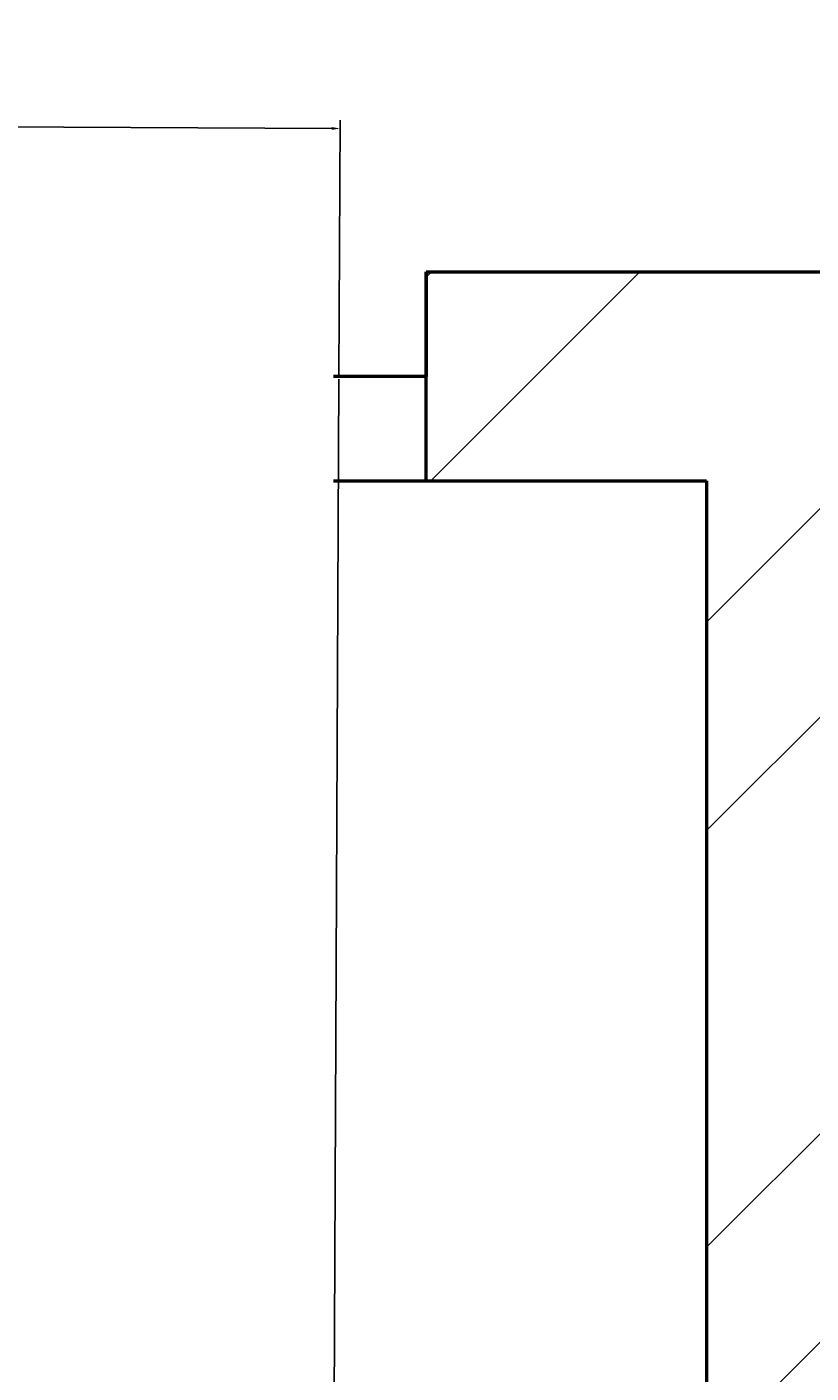
# Model space of a CAD drawing. Units: inches. Extents: x 1901 to 2863, y 888 to 2433.
# Tile 31 of 91: x 2590 to 2607, y 1376 to 1405. Entities that reach past the tile are written whole.
import ezdxf

# ---------------------------------------------------------------- set-up
doc = ezdxf.new("R2010")
doc.units = ezdxf.units.IN
for name, color, linetype, lineweight in [('A-ANNO-DIMS', 2, 'Continuous', 18), ('A-DOOR', 4, 'Continuous', 25), ('A-WALL', 7, 'Continuous', 50), ('A-WALL-PATT', 8, 'Continuous', 13)]:
    doc.layers.add(name, color=color, linetype=linetype, lineweight=lineweight)
doc.styles.get("Standard").update_dxf_attribs({"font": 'arial.ttf'})
doc.dimstyles.get("Standard").update_dxf_attribs({"dimtxt": 0.18, "dimasz": 0.18, "dimexe": 0.18, "dimexo": 0.0625, "dimgap": 0.09, "dimtad": 0, "dimtih": 1, "dimtoh": 1, "dimdec": 4, "dimzin": 0, "dimdsep": 46, "dimtxsty": 'Standard', "dimcen": 0.09, "dimadec": 0, "dimazin": 0, "dimtfac": 1, "dimtdec": 4, "dimtofl": 0, "dimtmove": 0, "dimatfit": 3, "dimfxl": 1, "dimtolj": 1, "dimtzin": 0, "dimarcsym": 0})

# ---------------------------------------------------------------- blocks, each defined once
blk = doc.blocks.new('DOOR-29')
blk.add_line((-0.004, -0.016), (-0.004, 35.984))
blk.add_arc((-0.004, 7.119), 28.865, 345.6888, 90)
blk = doc.blocks.new('*D32')
at = {"layer": 'A-ANNO-DIMS', "color": 0, "lineweight": -2, "transparency": 16777216}
for p, q in [((2566.833, 1398.027), (2566.858, 1403.544)), ((2567.038, 1403.364), (2581.416, 1403.297)), ((2596.85, 1403.225), (2582.472, 1403.292)), ((2597.005, 1397.887), (2597.03, 1403.404))]:
    blk.add_line(p, q, dxfattribs=at)
at = {"layer": 'A-ANNO-DIMS', "color": 0, "transparency": 16777216}
for points in [[(2567.038, 1403.394), (2567.037, 1403.334), (2566.858, 1403.364)], [(2596.85, 1403.255), (2596.849, 1403.195), (2597.03, 1403.224)]]:
    blk.add_solid(points, dxfattribs=at)
at = {"layer": 'Defpoints', "color": 0, "transparency": 16777216}
for p in [(2566.858, 1403.364), (2566.833, 1397.964), (2597.005, 1397.824)]:
    blk.add_point(p, dxfattribs=at)
at = {"layer": 'A-ANNO-DIMS', "color": 0, "transparency": 16777216, "insert": (2581.944, 1403.294), "char_height": 0.18, "attachment_point": 5}
blk.add_mtext('\\A1;30 TYP.', dxfattribs=at)

msp = doc.modelspace()

# ---------------------------------------------------------------- hatches: boundary and pattern name
at = {"layer": 'A-WALL-PATT'}
h = msp.add_hatch(dxfattribs=at)
h.set_pattern_fill('ANSI32', color=256)
h.paths.add_polyline_path([(2443.926, 2139.888), (2439.426, 2139.888), (2439.426, 2069.348), (2441.676, 2069.348), (2443.926, 2069.348), (2443.926, 2078.634), (2521.926, 2078.634), (2521.926, 2075.067), (2524.176, 2075.067), (2526.426, 2075.067), (2526.426, 2078.634), (2571.755, 2078.634), (2571.755, 2080.884), (2571.755, 2083.134), (2443.926, 2083.134)])
h.paths.add_polyline_path([(2526.426, 2054.634), (2524.176, 2054.634), (2521.926, 2054.634), (2521.926, 2030.634), (2443.926, 2030.634), (2443.926, 2045.348), (2439.426, 2045.348), (2439.426, 1983.867), (2443.926, 1983.867), (2443.926, 2026.134), (2521.926, 2026.134), (2526.426, 2026.134)])
h.paths.add_polyline_path([(2443.926, 1923.867), (2439.426, 1923.867), (2439.426, 1872.634), (2443.926, 1872.634)])
h.paths.add_polyline_path([(2636.233, 1766.134), (2609.926, 1766.134), (2609.926, 1779.785), (2605.426, 1779.785), (2605.426, 1766.134), (2486.614, 1766.134), (2486.614, 1770.671), (2482.114, 1770.671), (2482.114, 1766.134), (2482.114, 1761.634), (2636.233, 1761.634), (2636.233, 1763.884)])
h.paths.add_polyline_path([(2519.536, 1663.384), (2519.536, 1665.634), (2494.926, 1665.634), (2481.831, 1665.634), (2481.831, 1663.384), (2481.831, 1661.134), (2490.426, 1661.134), (2490.426, 1640.157), (2494.926, 1640.157), (2494.926, 1661.134), (2519.536, 1661.134)])
h.paths.add_polyline_path([(2443.926, 1712.134), (2443.926, 1716.634), (2414.464, 1716.634), (2414.464, 1712.134), (2439.426, 1712.134), (2439.426, 1545.507), (2443.926, 1545.507), (2443.926, 1661.134), (2448.475, 1661.134), (2448.475, 1665.634), (2443.926, 1665.634)])
h.paths.add_polyline_path([(2343.426, 1712.134), (2365.525, 1712.134), (2365.525, 1714.384), (2365.525, 1716.634), (2333.871, 1716.634), (2333.871, 1714.384), (2333.871, 1712.134), (2338.926, 1712.134), (2338.926, 1575.634), (2338.926, 1545.507), (2343.426, 1545.507), (2343.426, 1547.507), (2343.426, 1580.134)])
h.paths.add_polyline_path([(2752.926, 1665.634), (2579.536, 1665.634), (2579.536, 1661.134), (2615.926, 1661.134), (2615.926, 1529.134), (2598.931, 1529.134), (2598.931, 1524.634), (2623.127, 1524.634), (2623.127, 1526.884), (2623.127, 1529.134), (2620.426, 1529.134), (2620.426, 1661.134), (2748.426, 1661.134), (2748.426, 1633.499), (2752.926, 1633.499)])
h.paths.add_polyline_path([(2752.926, 1419.929), (2748.426, 1419.929), (2748.426, 1400.134), (2659.426, 1400.134), (2659.426, 1444.333), (2657.176, 1444.333), (2654.926, 1444.333), (2654.926, 1400.134), (2643.649, 1400.134), (2643.649, 1395.634), (2748.426, 1395.634), (2748.426, 1364.035), (2752.926, 1364.035)])
h.paths.add_polyline_path([(2752.926, 1492.878), (2748.426, 1492.878), (2748.426, 1476.634), (2667.426, 1476.634), (2667.426, 1479.71), (2665.176, 1479.71), (2662.926, 1479.71), (2662.926, 1476.634), (2654.926, 1476.634), (2654.926, 1469.536), (2659.426, 1469.536), (2659.426, 1472.134), (2748.426, 1472.134), (2748.426, 1455.929), (2752.926, 1455.929)])
h.paths.add_polyline_path([(2752.926, 1304.035), (2748.426, 1304.035), (2748.426, 1263.634), (2738.66, 1263.634), (2738.66, 1259.134), (2752.926, 1259.134)])
h.paths.add_polyline_path([(2685.926, 1259.134), (2695.49, 1259.134), (2695.49, 1261.384), (2695.49, 1263.634), (2677.837, 1263.634), (2677.837, 1261.384), (2677.837, 1259.134), (2681.426, 1259.134), (2681.426, 1203.634), (2653.277, 1203.634), (2653.277, 1199.134), (2685.926, 1199.134), (2685.926, 1203.634)])
h.paths.add_polyline_path([(2609.426, 1395.634), (2611.848, 1395.634), (2611.848, 1400.134), (2598.888, 1400.134), (2598.888, 1397.884), (2598.888, 1395.634), (2604.926, 1395.634), (2604.926, 1268.134), (2554.726, 1268.134), (2554.726, 1265.884), (2554.726, 1263.634), (2604.926, 1263.634), (2604.926, 1203.634), (2571.306, 1203.634), (2571.306, 1199.134), (2604.926, 1199.134), (2629.277, 1199.134), (2629.277, 1201.384), (2629.277, 1203.634), (2609.426, 1203.634), (2609.426, 1258.634), (2609.426, 1259.134), (2654.804, 1259.134), (2654.804, 1263.634), (2609.426, 1263.634)])
h.paths.add_polyline_path([(2443.926, 1304.035), (2439.426, 1304.035), (2439.426, 1259.134), (2443.926, 1259.134), (2456.16, 1259.134), (2456.16, 1261.384), (2456.16, 1263.634), (2443.926, 1263.634)])
h.paths.add_polyline_path([(2525.426, 1263.634), (2531.778, 1263.634), (2531.778, 1268.134), (2520.926, 1268.134), (2520.926, 1263.634), (2511.409, 1263.634), (2511.409, 1259.134), (2520.926, 1259.134), (2520.926, 1199.134), (2547.306, 1199.134), (2547.306, 1201.384), (2547.306, 1203.634), (2525.426, 1203.634)])
h.paths.add_polyline_path([(2443.926, 1434.842), (2439.426, 1434.842), (2439.426, 1364.035), (2441.676, 1364.035), (2443.926, 1364.035)])
h.paths.add_polyline_path([(2567.134, 1400.134), (2443.926, 1400.134), (2443.926, 1395.634), (2567.134, 1395.634)])
h.paths.add_polyline_path([(2443.926, 1545.507), (2439.426, 1545.507), (2439.426, 1494.842), (2443.926, 1494.842)])
h.paths.add_polyline_path([(2494.926, 1553.349), (2492.676, 1553.349), (2490.426, 1553.349), (2490.426, 1524.634), (2494.926, 1524.634), (2525.936, 1524.634), (2525.936, 1526.884), (2525.936, 1529.134), (2494.926, 1529.134)])
h.paths.add_polyline_path([(2752.926, 1573.499), (2748.426, 1573.499), (2748.426, 1529.134), (2657.759, 1529.134), (2657.759, 1524.634), (2662.926, 1524.634), (2662.926, 1498.631), (2667.426, 1498.631), (2667.426, 1524.634), (2748.426, 1524.634), (2748.426, 1516.878), (2752.926, 1516.878)])
h.paths.add_polyline_path([(2038.602, 2237.418), (2080.174, 2237.418), (2080.174, 2256.075), (2038.602, 2256.075)], flags=9)
h.paths.add_polyline_path([(2292.009, 1062.394), (2539.932, 1062.394), (2539.932, 1099.487), (2292.009, 1099.487)], flags=9)
h.paths.add_polyline_path([(2424.91, 1832.253), (2448.513, 1832.253), (2448.513, 1846.678), (2424.91, 1846.678)], flags=9)
h.paths.add_polyline_path([(2359.076, 1832.253), (2382.678, 1832.253), (2382.678, 1846.678), (2359.076, 1846.678)], flags=9)
h.paths.add_polyline_path([(2352.899, 1684.802), (2367.543, 1684.802), (2367.543, 1697.167), (2352.899, 1697.167)], flags=9)
h.paths.add_polyline_path([(2079.288, 1755.826), (2169.024, 1755.826), (2169.024, 1774.372), (2079.288, 1774.372)], flags=9)
h.paths.add_polyline_path([(2404.09, 1373.857), (2404.09, 1463.593), (2385.544, 1463.593), (2385.544, 1373.857)], flags=9)
h.paths.add_polyline_path([(2268.091, 2236.371), (2309.636, 2236.371), (2309.636, 2255.028), (2268.091, 2255.028)], flags=9)
h.paths.add_polyline_path([(2575.96, 1700.951), (2665.696, 1700.951), (2665.696, 1719.498), (2575.96, 1719.498)], flags=9)
h.paths.add_polyline_path([(2302.962, 1878.474), (2329.524, 1878.474), (2329.524, 1888.777), (2302.962, 1888.777)], flags=9)
h.paths.add_polyline_path([(2097.415, 2240.576), (2126.573, 2240.576), (2126.573, 2259.233), (2097.415, 2259.233)], flags=9)
h.paths.add_polyline_path([(2208.725, 2246.124), (2237.882, 2246.124), (2237.882, 2264.781), (2208.725, 2264.781)], flags=9)
h.paths.add_polyline_path([(2038.147, 1925.958), (2076.987, 1925.958), (2076.987, 1944.615), (2038.147, 1944.615)], flags=9)
h.paths.add_polyline_path([(2239.144, 1926.672), (2288.465, 1926.672), (2288.465, 1945.329), (2239.144, 1945.329)], flags=9)
h.paths.add_polyline_path([(2175.429, 2007.33), (2212.356, 2007.33), (2212.356, 2025.987), (2175.429, 2025.987)], flags=9)
h.paths.add_polyline_path([(2225.034, 2091.794), (2263.875, 2091.794), (2263.875, 2110.451), (2225.034, 2110.451)], flags=9)
h.paths.add_polyline_path([(2035.398, 2098.478), (2074.238, 2098.478), (2074.238, 2117.135), (2035.398, 2117.135)], flags=9)
h.paths.add_polyline_path([(2050.102, 2029.209), (2083.26, 2029.209), (2083.26, 2047.866), (2050.102, 2047.866)], flags=9)
h.paths.add_polyline_path([(2069.677, 1956.719), (2098.835, 1956.719), (2098.835, 1975.376), (2069.677, 1975.376)], flags=9)
h.paths.add_polyline_path([(2328.62, 1753.336), (2361.663, 1753.336), (2361.663, 1771.993), (2328.62, 1771.993)], flags=9)
h.paths.add_polyline_path([(2395.162, 2060.888), (2395.162, 2140.654), (2378.676, 2140.654), (2378.676, 2060.888)], flags=9)
h.paths.add_polyline_path([(2463.728, 2059.02), (2492.886, 2059.02), (2492.886, 2077.677), (2463.728, 2077.677)], flags=9)
h.paths.add_polyline_path([(2458.027, 2181.536), (2496.868, 2181.536), (2496.868, 2200.194), (2458.027, 2200.194)], flags=9)
h.paths.add_polyline_path([(2456.855, 2228.831), (2498.401, 2228.831), (2498.401, 2247.488), (2456.855, 2247.488)], flags=9)
h.paths.add_polyline_path([(2527.577, 2243.074), (2556.735, 2243.074), (2556.735, 2261.731), (2527.577, 2261.731)], flags=9)
h.paths.add_polyline_path([(2694.461, 2232.767), (2736.033, 2232.767), (2736.033, 2251.425), (2694.461, 2251.425)], flags=9)
h.paths.add_polyline_path([(2637.821, 2249.225), (2666.979, 2249.225), (2666.979, 2267.882), (2637.821, 2267.882)], flags=9)
h.paths.add_polyline_path([(2623.687, 2183.541), (2662.528, 2183.541), (2662.528, 2202.199), (2623.687, 2202.199)], flags=9)
h.paths.add_polyline_path([(2691.965, 2021.5), (2725.124, 2021.5), (2725.124, 2040.157), (2691.965, 2040.157)], flags=9)
h.paths.add_polyline_path([(2621.043, 1975.912), (2662.335, 1975.912), (2662.335, 1994.569), (2621.043, 1994.569)], flags=9)
h.paths.add_polyline_path([(2479.032, 1927.62), (2519.844, 1927.62), (2519.844, 1946.277), (2479.032, 1946.277)], flags=9)
h.paths.add_polyline_path([(2670.941, 1849.076), (2716.005, 1849.076), (2716.005, 1867.734), (2670.941, 1867.734)], flags=9)
h.paths.add_polyline_path([(2523.613, 1782.956), (2550.175, 1782.956), (2550.175, 1793.26), (2523.613, 1793.26)], flags=9)
h.paths.add_polyline_path([(2450.841, 1207.331), (2492.386, 1207.331), (2492.386, 1225.989), (2450.841, 1225.989)], flags=9)
h.paths.add_polyline_path([(2527.751, 1203.841), (2556.908, 1203.841), (2556.908, 1222.499), (2527.751, 1222.499)], flags=9)
h.paths.add_polyline_path([(2639.111, 1207.2), (2668.268, 1207.2), (2668.268, 1225.857), (2639.111, 1225.857)], flags=9)
h.paths.add_polyline_path([(2692.594, 1218.965), (2734.167, 1218.965), (2734.167, 1237.623), (2692.594, 1237.623)], flags=9)
h.paths.add_polyline_path([(2669.266, 1366.329), (2708.106, 1366.329), (2708.106, 1384.987), (2669.266, 1384.987)], flags=25)
h.paths.add_polyline_path([(2463.313, 1358.031), (2502.153, 1358.031), (2502.153, 1376.688), (2463.313, 1376.688)], flags=9)
h.paths.add_polyline_path([(2494.725, 1449.963), (2531.652, 1449.963), (2531.652, 1468.62), (2494.725, 1468.62)], flags=9)
h.paths.add_polyline_path([(2675.565, 1422.157), (2708.724, 1422.157), (2708.724, 1440.815), (2675.565, 1440.815)], flags=25)
h.paths.add_polyline_path([(2685.634, 1493.891), (2714.792, 1493.891), (2714.792, 1512.548), (2685.634, 1512.548)], flags=9)
h.paths.add_polyline_path([(2686.805, 1529.913), (2725.645, 1529.913), (2725.645, 1548.57), (2686.805, 1548.57)], flags=25)
h.paths.add_polyline_path([(2503.651, 1537.991), (2552.972, 1537.991), (2552.972, 1556.648), (2503.651, 1556.648)], flags=9)
h.paths.add_polyline_path([(2291.713, 1643.504), (2318.275, 1643.504), (2318.275, 1653.807), (2291.713, 1653.807)], flags=9)
h.paths.add_polyline_path([(2450.626, 1610.52), (2477.189, 1610.52), (2477.189, 1620.824), (2450.626, 1620.824)], flags=9)
h.paths.add_polyline_path([(2359.985, 1551.814), (2422.253, 1551.814), (2422.253, 1562.117), (2359.985, 1562.117)], flags=9)
h.paths.add_polyline_path([(2280.106, 1249.006), (2321.651, 1249.006), (2321.651, 1267.663), (2280.106, 1267.663)], flags=9)
h.paths.add_polyline_path([(2164.057, 1274.232), (2193.215, 1274.232), (2193.215, 1292.889), (2164.057, 1292.889)], flags=9)
h.paths.add_polyline_path([(2118.21, 1277.694), (2151.252, 1277.694), (2151.252, 1296.351), (2118.21, 1296.351)], flags=9)
h.paths.add_polyline_path([(2031.946, 1268.529), (2073.519, 1268.529), (2073.519, 1287.187), (2031.946, 1287.187)], flags=9)
h.paths.add_polyline_path([(2050.199, 1409.079), (2089.04, 1409.079), (2089.04, 1427.736), (2050.199, 1427.736)], flags=9)
h.paths.add_polyline_path([(2243.743, 1421.032), (2282.584, 1421.032), (2282.584, 1439.689), (2243.743, 1439.689)], flags=9)
h.paths.add_polyline_path([(2190.746, 1509.769), (2231.558, 1509.769), (2231.558, 1528.426), (2190.746, 1528.426)], flags=9)
h.paths.add_polyline_path([(2058.392, 1475.415), (2091.55, 1475.415), (2091.55, 1494.073), (2058.392, 1494.073)], flags=9)
h.paths.add_polyline_path([(2062.447, 1553.09), (2091.605, 1553.09), (2091.605, 1571.747), (2062.447, 1571.747)], flags=9)
h.paths.add_polyline_path([(2219.524, 1590.365), (2266.147, 1590.365), (2266.147, 1609.022), (2219.524, 1609.022)], flags=9)
h.paths.add_polyline_path([(2041.072, 1584.188), (2079.912, 1584.188), (2079.912, 1602.845), (2041.072, 1602.845)], flags=9)

# ---------------------------------------------------------------- linework, layer by layer
at = {"layer": 'A-WALL'}
for p, q in [((2598.888, 1395.634), (2598.888, 1400.134)), ((2598.888, 1400.134), (2598.888, 1397.884)), ((2598.888, 1400.134), (2611.848, 1400.134)), ((2598.888, 1397.884), (2596.888, 1397.884)), ((2596.888, 1395.634), (2604.926, 1395.634)), ((2604.926, 1395.634), (2604.926, 1268.134))]:
    msp.add_line(p, q, dxfattribs=at)

# ---------------------------------------------------------------- block references
at = {"layer": 'A-DOOR', "rotation": 179.7338121645225}
msp.add_blockref('DOOR-29', (2597.001, 1397.808), dxfattribs=at)

# ---------------------------------------------------------------- dimensions: what is measured, and where the dimension line sits
at = {"layer": 'A-ANNO-DIMS'}
dim = msp.add_linear_dim(base=(2566.858, 1403.364), p1=(2597.005, 1397.824), p2=(2566.833, 1397.964), angle=179.7338, text='<> TYP.', dimstyle='Standard', override={"dimdec": 0, "dimlfac": 1, "dimrnd": 0, "dimzin": 0, "dimdsep": 46, "dimlunit": 2}, dxfattribs=at)
dim.commit()
dim.dimension.update_dxf_attribs({"geometry": '*D32', "text_midpoint": (2581.944, 1403.294)})

doc.saveas('drawing.dxf')
